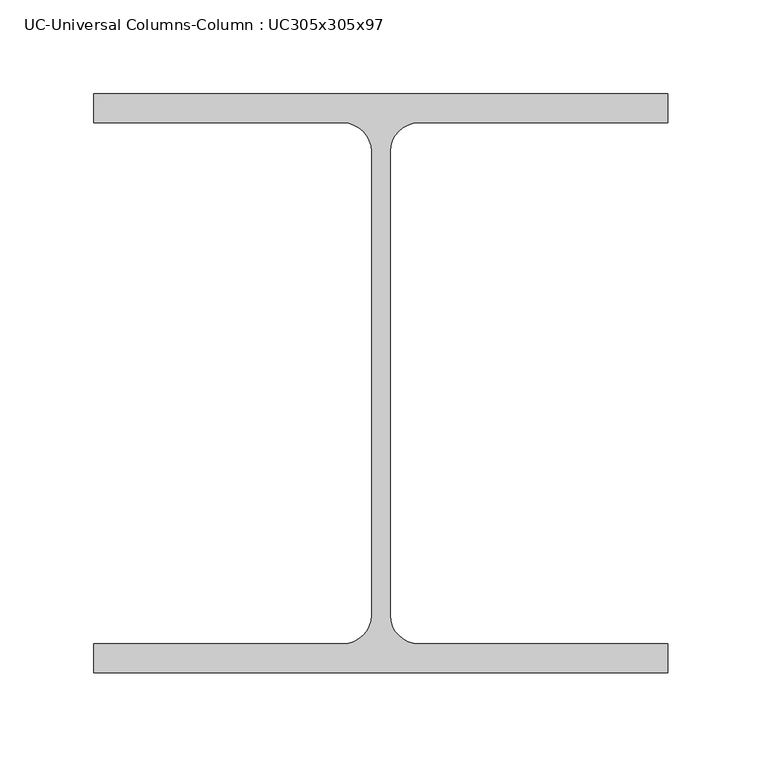
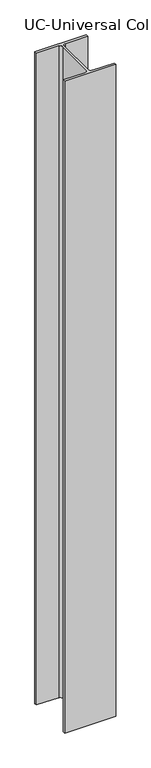
"""IFC4 building model written with IfcOpenShell, lengths in millimetres: column geometry, UC-Universal Columns-Column : UC305x305x97."""

from ifc_helpers import new_model, si_unit, point, frame, frame_2d, origin, place, context, project, spatial, polyline, circle_curve, trimmed, segment, composite_curve, outline, extrude, source, transform, mapped, element, save


def uc_universal_columns_column_uc305x305x97_28816581(model_context):
    return source(origin(), model_context, "Body", "SweptSolid", [
        extrude(outline(composite_curve([segment(polyline([(152.65, 153.95), (152.65, 138.55), (20.15, 138.55)]), True, "CONTINUOUS"), segment(trimmed(circle_curve(frame_2d((20.15, 123.35)), 15.2), [point((20.15, 138.55))], [point((4.95, 123.35))], True, "CARTESIAN"), True, "CONTINUOUS"), segment(polyline([(4.95, 123.35), (4.95, -123.35)]), True, "CONTINUOUS"), segment(trimmed(circle_curve(frame_2d((20.15, -123.35)), 15.2), [point((4.95, -123.35))], [point((20.15, -138.55))], True, "CARTESIAN"), True, "CONTINUOUS"), segment(polyline([(20.15, -138.55), (152.65, -138.55), (152.65, -153.95), (-152.65, -153.95), (-152.65, -138.55), (-20.15, -138.55)]), True, "CONTINUOUS"), segment(trimmed(circle_curve(frame_2d((-20.15, -123.35)), 15.2), [point((-20.15, -138.55))], [point((-4.95, -123.35))], True, "CARTESIAN"), True, "CONTINUOUS"), segment(polyline([(-4.95, -123.35), (-4.95, 123.35)]), True, "CONTINUOUS"), segment(trimmed(circle_curve(frame_2d((-20.15, 123.35)), 15.2), [point((-4.95, 123.35))], [point((-20.15, 138.55))], True, "CARTESIAN"), True, "CONTINUOUS"), segment(polyline([(-20.15, 138.55), (-152.65, 138.55), (-152.65, 153.95), (152.65, 153.95)]), True, "CONTINUOUS")], self_intersect=False)), frame((0.0, 0.0, -1812.3304639), z_axis=(0.0, 0.0, 1.0), x_axis=(1.0, 0.0, 0.0)), (0.0, 0.0, 1.0), 4114.6),
    ])


if __name__ == "__main__":
    model = new_model("IFC4")
    model_context = context("Model", 3, world=origin())
    ifc_project = project(units=[si_unit("LENGTHUNIT", "METRE", prefix="MILLI")], contexts=[model_context])
    site = spatial("IfcSite", under=ifc_project)
    building = spatial("IfcBuilding", under=site)
    placement = place(None, origin())
    uc_universal_columns_column_uc305x305x97_shape = uc_universal_columns_column_uc305x305x97_28816581(model_context)
    element("IfcColumn", 1, ObjectType="UC-Universal Columns-Column : UC305x305x97", at=placement, inside=building, context=model_context, shape_type="MappedRepresentation", body=[
        mapped(uc_universal_columns_column_uc305x305x97_shape, transform((0.0, 0.0, 0.0), x_axis=(1.0, 0.0, 0.0), y_axis=(0.0, 1.0, 0.0), z_axis=(0.0, 0.0, 1.0))),
    ])
    save(model, "model.ifc")

# Revit data of these elements
# Type "UC-Universal Columns-Column : UC305x305x97"
#   Section Name Key = "UC305x305x97"
#   Width = 30.53 cm
#   Web Thickness = 0.99 cm
#   Web Fillet = 1.52 cm
#   Warping Constant = 1560000.0 cm⁶
#   Torsional Moment of Inertia = 91.20 cm⁴
#   Section Area = 123.0 cm²
#   Plastic Modulus weak axis = 726.0 cm³
#   Plastic Modulus strong axis = 1592.0 cm³
#   Nominal Weight = 96.8996 kgf/m
#   Moment of Inertia weak axis = 7308.00 cm⁴
#   Moment of Inertia strong axis = 22249.00 cm⁴
#   Height = 30.79 cm
#   Flange Thickness = 1.54 cm
#   Elastic Modulus weak axis = 479.0 cm³
#   Elastic Modulus strong axis = 1445.0 cm³
#   Centroid Vertical = 15.395 cm
#   Centroid Horizontal = 15.265 cm
#   Bolt Spacing = 14.0 cm
#   Structural Material [instance default] = Metal - Steel 43-275
#   Type Comments = ""
#   Assembly Code = ""
# Element 1 (IfcColumn, "UC-Universal Columns-Column : UC305x305x97")
#   Materials on its faces: "Metal - Steel 43-275"
# Materials
#   "Metal - Steel 43-275": class "Metal", colour RGB 247 247 247, transparency 0, Cost = 0
